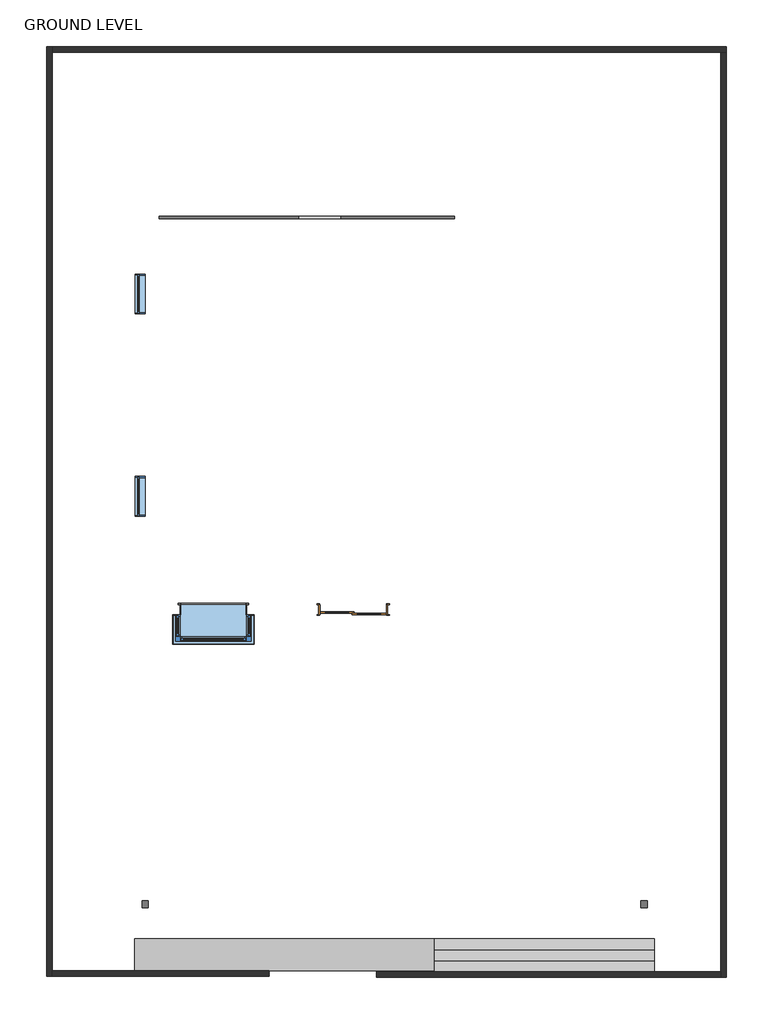
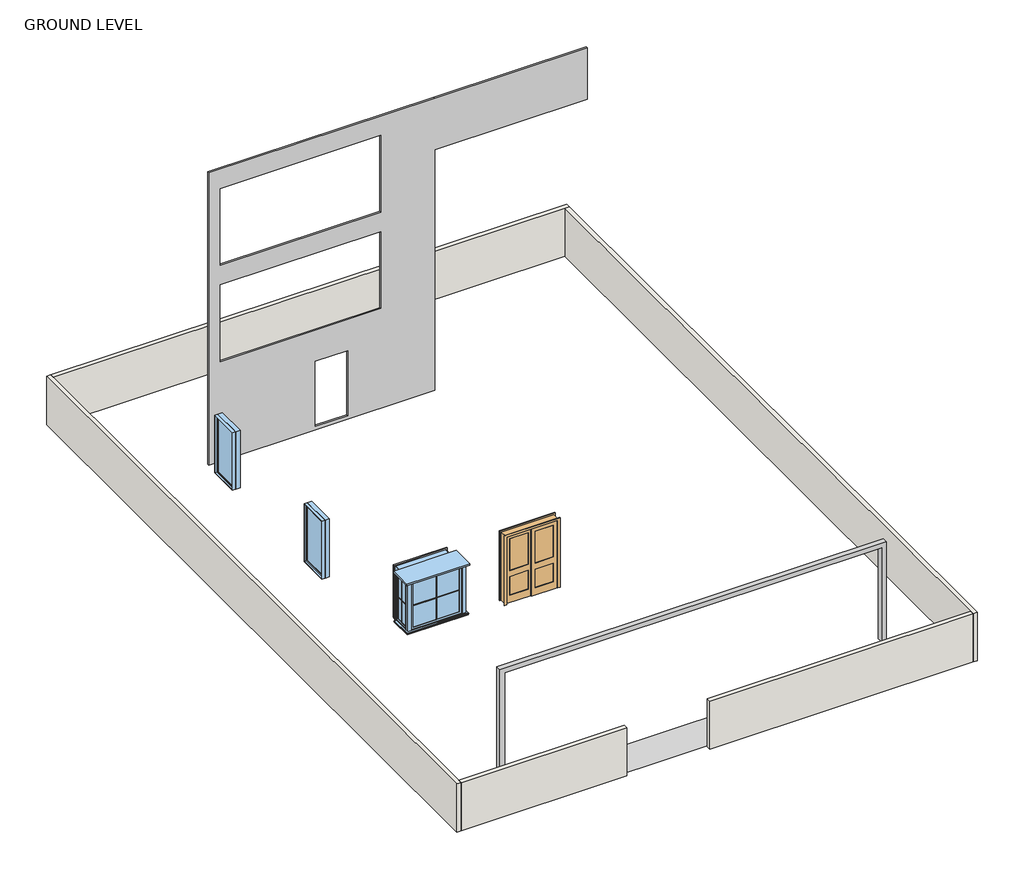
# One storey: 8 proxies, 5 walls, 3 windows, 1 door.
"""IFC4 building model written with IfcOpenShell, lengths in millimetres."""

from ifc_helpers import new_model, si_unit, origin, origin_with_axes, place, context, project, spatial, polyline, outline, extrude, faceted_brep, transform, mapped, element, save
from components import generic_models_11_generic_models_11_747a53b2, generic_models_19_generic_models_19_d8e6bd8f, generic_models_30_generic_models_30_d6d6d2d1, generic_models_31_generic_models_31_aad501af, muntin_pattern_2x2_muntin_pattern_2x2_eeef18e2, muntin_pattern_2x2_muntin_pattern_2x2_218eda85, trim_window_interior_flat_picture_frame_524b5c54, door_2b3f2951, window_2e8ca8a3, window_dda79932

model = new_model("IFC4")

# Units and contexts
model_context = context("Model", 3, world=origin())
ifc_project = project(units=[si_unit("LENGTHUNIT", "METRE", prefix="MILLI")], contexts=[model_context])

# Site, building, storey
site = spatial("IfcSite", under=ifc_project)
building = spatial("IfcBuilding", under=site)
storey = spatial("IfcBuildingStorey", under=building, Name="GROUND LEVEL", Elevation=0.0)

# Proxies
placement = place(None, origin())
generic_models_11_generic_models_11_shape = generic_models_11_generic_models_11_747a53b2(model_context)
element("IfcBuildingElementProxy", 1, Name="Generic Models 11 : Generic Models 11", ObjectType="Generic Models 11 : Generic Models 11", at=placement, inside=storey, context=model_context, shape_type="MappedRepresentation", body=[
    mapped(generic_models_11_generic_models_11_shape, transform((0.0, 0.0, 0.0), x_axis=(1.0, 0.0, 0.0), y_axis=(0.0, 1.0, 0.0), z_axis=(0.0, 0.0, 1.0))),
])
generic_models_19_generic_models_19_shape = generic_models_19_generic_models_19_d8e6bd8f(model_context)
element("IfcBuildingElementProxy", 2, Name="Generic Models 19 : Generic Models 19", ObjectType="Generic Models 19 : Generic Models 19", at=placement, inside=storey, context=model_context, shape_type="MappedRepresentation", body=[
    mapped(generic_models_19_generic_models_19_shape, transform((0.0, 0.0, 0.0), x_axis=(1.0, 0.0, 0.0), y_axis=(0.0, 1.0, 0.0), z_axis=(0.0, 0.0, 1.0))),
])
generic_models_30_generic_models_30_shape = generic_models_30_generic_models_30_d6d6d2d1(model_context)
element("IfcBuildingElementProxy", 3, Name="Generic Models 30 : Generic Models 30", ObjectType="Generic Models 30 : Generic Models 30", at=placement, inside=storey, context=model_context, shape_type="MappedRepresentation", body=[
    mapped(generic_models_30_generic_models_30_shape, transform((0.0, 0.0, 0.0), x_axis=(1.0, 0.0, 0.0), y_axis=(0.0, 1.0, 0.0), z_axis=(0.0, 0.0, 1.0))),
])
generic_models_31_generic_models_31_shape = generic_models_31_generic_models_31_aad501af(model_context)
element("IfcBuildingElementProxy", 4, Name="Generic Models 31 : Generic Models 31", ObjectType="Generic Models 31 : Generic Models 31", at=placement, inside=storey, context=model_context, shape_type="MappedRepresentation", body=[
    mapped(generic_models_31_generic_models_31_shape, transform((0.0, 0.0, 0.0), x_axis=(1.0, 0.0, 0.0), y_axis=(0.0, 1.0, 0.0), z_axis=(0.0, 0.0, 1.0))),
])
muntin_pattern_2x2_muntin_pattern_2x2_shape = muntin_pattern_2x2_muntin_pattern_2x2_eeef18e2(model_context)
element("IfcBuildingElementProxy", 5, Name="Muntin Pattern_2x2 : Muntin Pattern_2x2", ObjectType="Muntin Pattern_2x2 : Muntin Pattern_2x2", at=placement, inside=storey, context=model_context, shape_type="MappedRepresentation", body=[
    mapped(muntin_pattern_2x2_muntin_pattern_2x2_shape, transform((-8201.8781265, -1299.9392532, 730.25), x_axis=(-1.0, 0.0, 0.0), y_axis=(0.0, -1.0, 0.0), z_axis=(0.0, 0.0, 1.0))),
])
muntin_pattern_2x2_muntin_pattern_2x2_2_shape = muntin_pattern_2x2_muntin_pattern_2x2_218eda85(model_context)
element("IfcBuildingElementProxy", 6, Name="Muntin Pattern_2x2 : Muntin Pattern_2x2", ObjectType="Muntin Pattern_2x2 : Muntin Pattern_2x2", at=placement, inside=storey, context=model_context, shape_type="MappedRepresentation", body=[
    mapped(muntin_pattern_2x2_muntin_pattern_2x2_2_shape, transform((-7379.5531265, -985.6142532, 730.25), x_axis=(0.0, 1.0, 0.0), y_axis=(-1.0, 0.0, 0.0), z_axis=(0.0, 0.0, 1.0))),
])
element("IfcBuildingElementProxy", 7, Name="Muntin Pattern_2x2 : Muntin Pattern_2x2", ObjectType="Muntin Pattern_2x2 : Muntin Pattern_2x2", at=placement, inside=storey, context=model_context, shape_type="MappedRepresentation", body=[
    mapped(muntin_pattern_2x2_muntin_pattern_2x2_2_shape, transform((-9024.2031265, -985.6142532, 730.25), x_axis=(0.0, -1.0, 0.0), y_axis=(1.0, 0.0, 0.0), z_axis=(0.0, 0.0, 1.0))),
])
trim_window_interior_flat_picture_frame_shape = trim_window_interior_flat_picture_frame_524b5c54(model_context)
element("IfcBuildingElementProxy", 8, Name="Trim-Window-Interior-Flat : Picture Frame", ObjectType="Trim-Window-Interior-Flat : Picture Frame", at=placement, inside=storey, context=model_context, shape_type="MappedRepresentation", body=[
    mapped(trim_window_interior_flat_picture_frame_shape, transform((-8201.8781265, -503.0142532, 2184.4), x_axis=(-1.0, 0.0, 0.0), y_axis=(0.0, 0.0, 1.0), z_axis=(0.0, 1.0, 0.0))),
])

# Door
door_shape = door_2b3f2951(model_context)
element("IfcDoor", 9, ObjectType="Door-Interior-Double-Sliding-2_Panel-Wood : 60\" x 84\"", at=placement, inside=storey, context=model_context, shape_type="MappedRepresentation", body=[
    mapped(door_shape, transform((-5001.4781265, -620.4892532, 0.0), x_axis=(-1.0, 0.0, 0.0), y_axis=(0.0, -1.0, 0.0), z_axis=(0.0, 0.0, 1.0))),
])

# Walls
element("IfcWall", 10, ObjectType="parapet wall 5\"", at=placement, inside=storey, context=model_context, shape_type="Brep", body=[
    faceted_brep([(-11897.5781265, -9005.1279205, 0.0), (-11897.5781265, -8878.1279205, 0.0), (-11897.5781265, 12146.1857468, 0.0), (-11897.5781265, 12273.1857468, 0.0), (-11897.5781265, 12273.1857468, 1524.0), (-11897.5781265, 12146.1857468, 1524.0), (-11897.5781265, -8878.1279205, 1524.0), (-11897.5781265, -9005.1279205, 1524.0), (-12024.5781265, -9005.1279205, 0.0), (-12024.5781265, -9005.1279205, 1524.0), (-12024.5781265, 12273.1857468, 1524.0), (-12024.5781265, 12273.1857468, 0.0)], [[[0, 1, 2, 3, 4, 5, 6, 7]], [[8, 9, 10, 11]], [[3, 2, 1, 0, 8, 11]], [[7, 6, 5, 4, 10, 9]], [[4, 3, 11, 10]], [[0, 7, 9, 8]]]),
])
element("IfcWall", 11, ObjectType="parapet wall 5\"", at=placement, inside=storey, context=model_context, shape_type="Brep", body=[
    faceted_brep([(-11897.5781265, 12146.1857468, 0.0), (3418.6218735, 12146.1857468, 0.0), (3545.6218735, 12146.1857468, 0.0), (3545.6218735, 12146.1857468, 1524.0), (3418.6218735, 12146.1857468, 1524.0), (-11897.5781265, 12146.1857468, 1524.0), (-11897.5781265, 12273.1857468, 0.0), (-11897.5781265, 12273.1857468, 1524.0), (3545.6218735, 12273.1857468, 1524.0), (3545.6218735, 12273.1857468, 0.0)], [[[0, 1, 2, 3, 4, 5]], [[6, 7, 8, 9]], [[2, 1, 0, 6, 9]], [[5, 4, 3, 8, 7]], [[0, 5, 7, 6]], [[3, 2, 9, 8]]]),
])
element("IfcWall", 12, ObjectType="parapet wall 5\"", at=placement, inside=storey, context=model_context, shape_type="Brep", body=[
    faceted_brep([(3418.6218735, 12146.1857468, 0.0), (3418.6218735, -8909.9432518, 0.0), (3418.6218735, -9036.9432518, 0.0), (3418.6218735, -9036.9432518, 1524.0), (3418.6218735, -8909.9432518, 1524.0), (3418.6218735, 12146.1857468, 1524.0), (3545.6218735, 12146.1857468, 0.0), (3545.6218735, 12146.1857468, 1524.0), (3545.6218735, -9036.9432518, 1524.0), (3545.6218735, -9036.9432518, 0.0)], [[[0, 1, 2, 3, 4, 5]], [[6, 7, 8, 9]], [[2, 1, 0, 6, 9]], [[5, 4, 3, 8, 7]], [[0, 5, 7, 6]], [[3, 2, 9, 8]]]),
])
element("IfcWall", 13, ObjectType="parapet wall 5\"", at=placement, inside=storey, context=model_context, shape_type="SweptSolid", body=[
    extrude(outline(polyline([(-4468.0781265, -8909.9432518), (3418.6218735, -8909.9432518), (3418.6218735, -9036.9432518), (-4468.0781265, -9036.9432518), (-4468.0781265, -8909.9432518)])), origin_with_axes(), (0.0, 0.0, 1.0), 1524.0),
])
element("IfcWall", 14, ObjectType="parapet wall 5\"", at=placement, inside=storey, context=model_context, shape_type="SweptSolid", body=[
    extrude(outline(polyline([(-11897.5781265, -8878.1279205), (-6931.8781265, -8878.1279205), (-6931.8781265, -9005.1279205), (-11897.5781265, -9005.1279205), (-11897.5781265, -8878.1279205)])), origin_with_axes(), (0.0, 0.0, 1.0), 1524.0),
])

# Windows
window_shape = window_2e8ca8a3(model_context)
element("IfcWindow", 15, ObjectType="Fixed : window 3' x 6\"", at=placement, inside=storey, context=model_context, shape_type="MappedRepresentation", body=[
    mapped(window_shape, transform((-9878.2781265, 6647.0857468, 0.0), x_axis=(0.0, 1.0, 0.0), y_axis=(-1.0, 0.0, 0.0), z_axis=(0.0, 0.0, 1.0))),
])
element("IfcWindow", 16, ObjectType="Fixed : window 3' x 6\"", at=placement, inside=storey, context=model_context, shape_type="MappedRepresentation", body=[
    mapped(window_shape, transform((-9878.2781265, 2011.5857468, 0.0), x_axis=(0.0, 1.0, 0.0), y_axis=(-1.0, 0.0, 0.0), z_axis=(0.0, 0.0, 1.0))),
])
window_2_shape = window_dda79932(model_context)
element("IfcWindow", 17, ObjectType="Window-Bay-Casement-Box-90_Degree_Angle-Center_Fixed : 60\" x 60\" x 24\"", at=placement, inside=storey, context=model_context, shape_type="MappedRepresentation", body=[
    mapped(window_2_shape, transform((-8201.8781265, -617.3142532, 0.0), x_axis=(-1.0, 0.0, 0.0), y_axis=(0.0, -1.0, 0.0), z_axis=(0.0, 0.0, 1.0))),
])

save(model, "model.ifc")

# Revit data of these elements
# Type "Muntin Pattern_2x2 : Muntin Pattern_2x2"
#   Width [instance default] = 4' - 0"
#   Thickness = 0' - 0 1/2"
#   Height [instance default] = 4' - 0"
#   Distance = 0' - 0 3/4"
#   Interior Material [instance default] = none
#   Exterior Material [instance default] = none
#   Default Elevation = 0
# Type "Trim-Window-Interior-Flat : Picture Frame"
#   Trim Thickness_Picture Frame = 0' - 1 1/4"
#   Trim Width = 0' - 2 1/4"
#   Trim Thickness_with Sill = 0' - 0 3/4"
#   Sill Thickness = 0' - 1 1/4"
#   Opening Width [instance default] = 2' - 0"
#   Opening Height [instance default] = 3' - 0"
#   Default Elevation = 4' - 0"
#   Sill = no
#   Picture Frame = yes
#   Trim Material [instance default] = none
# Type "Door-Interior-Double-Sliding-2_Panel-Wood : 60\" x 84\""
#   Type Mark = "10"
#   Assembly Code = "C1020300"
#   Analytic Construction = "Wooden"
#   Top Rail = 0' - 4 11/16"
#   Thickness = 0' - 1 3/8"
#   Thermal Resistance (R) = 2.5876 (h·ft²·°F)/BTU
#   Stiles = 0' - 4 3/4"
#   Rough Width = 5' - 2"
#   Rough Height = 7' - 1"
#   Lock Rail = 0' - 7 1/2"
#   Height = 7' - 0"
#   Width = 5' - 0"
#   Heat Transfer Coefficient (U) = 0.3865 BTU/(h·ft²·°F)
#   Bottom Rail = 0' - 9 1/8"
#   Trim Material = Cherry
#   Panel Material = Cherry
#   Frame Material = Cherry
#   Visual Light Transmittance = 0
#   Solar Heat Gain Coefficient = 0
#   Wall Closure = (empty or 0)
#   Function = (empty or 0)
# Type "parapet wall 5\""
#   Assembly Code = "B2010"
# Type "Fixed : window 3' x 6\""
#   Type Mark = "26"
#   Construction Type Id = "GSP4R"
#   Assembly Code = "B2020100"
#   Analytic Construction = "1/8 in Pilkington single glazing"
#   Visual Light Transmittance = 0.9
#   Solar Heat Gain Coefficient = 0.78
#   Heat Transfer Coefficient (U) = 0.6496 BTU/(h·ft²·°F)
#   Height = 6' - 0"
#   Default Sill Height = 3' - 0"
#   Width = 3' - 0"
#   Window Inset = 0' - 2"
#   Define Thermal Properties by = 1
#   Glass Pane Material = Glass
#   Sash Material = Sash
#   Wall Closure = (empty or 0)
# Type "Window-Bay-Casement-Box-90_Degree_Angle-Center_Fixed : 60\" x 60\" x 24\""
#   Type Mark = "29"
#   Fire Rating = "0.5h"
#   Assembly Code = "B2020100"
#   Analytic Construction = "1/8 in Pilkington single glazing"
#   Width = 5' - 0"
#   Wall Thickness [instance default] = 0' - 6"
#   Visual Light Transmittance = 0.9
#   Trim Width = 5' - 8"
#   Trim Height = 5' - 0"
#   Thermal Resistance (R) = 1.5394 (h·ft²·°F)/BTU
#   Solar Heat Gain Coefficient = 0.86
#   Rough Width = 5' - 0 1/2"
#   Rough Height = 5' - 0 1/2"
#   Height 1 = 5' - 2"
#   Height = 5' - 0"
#   Heat Transfer Coefficient (U) = 0.6496 BTU/(h·ft²·°F)
#   Depth = 2' - 0"
#   Default Sill Height = 2' - 0"
#   Side Muntin Visibility = yes
#   Center Muntin Visibility = yes
#   Interior Trim Visibility [instance default] = yes
#   Exterior Trim Visibility [instance default] = yes
#   Side Muntin Pattern = Muntin Pattern_2x2 : Muntin Pattern_2x2
#   Center Muntin Pattern = Muntin Pattern_2x2 : Muntin Pattern_2x2
#   Interior Trim Material = Wood - Stained
#   Exterior Trim Material = Clad - White
#   Exterior Trim = element 424880
#   Interior Trim = Trim-Window-Interior-Flat : Picture Frame
#   Interior Frame Material = Wood - Stained
#   Glass Panel Material = Glass
#   Exterior Frame Material = Clad - White
#   Wall Closure = (empty or 0)
# Element 1 (IfcBuildingElementProxy, "Generic Models 11 : Generic Models 11")
#   Phase Created = New Construction
# Element 2 (IfcBuildingElementProxy, "Generic Models 19 : Generic Models 19")
#   Phase Created = New Construction
# Element 3 (IfcBuildingElementProxy, "Generic Models 30 : Generic Models 30")
#   Phase Created = New Construction
# Element 4 (IfcBuildingElementProxy, "Generic Models 31 : Generic Models 31")
#   Phase Created = New Construction
# Element 5 (IfcBuildingElementProxy, "Muntin Pattern_2x2 : Muntin Pattern_2x2")
#   Width = 4' - 6 1/2"
#   Height = 4' - 6 1/2"
#   Interior Material = Wood - Stained
#   Exterior Material = Clad - White
#   Phase Created = New Construction
#   Materials on its faces: "Clad - White", "Wood - Stained"
# Elements 6, 7 (IfcBuildingElementProxy, "Muntin Pattern_2x2 : Muntin Pattern_2x2")
#   Width = 1' - 2 1/2"
#   Height = 4' - 6 1/2"
#   Interior Material = Wood - Stained
#   Exterior Material = Clad - White
#   Phase Created = New Construction
#   Materials on its faces: "Clad - White", "Wood - Stained"
# Element 8 (IfcBuildingElementProxy, "Trim-Window-Interior-Flat : Picture Frame")
#   Opening Width = 5' - 0"
#   Opening Height = 5' - 2"
#   Trim Material = Wood - Stained
#   Phase Created = New Construction
#   Materials on its faces: "Wood - Stained"
# Element 9 (IfcDoor, "Door-Interior-Double-Sliding-2_Panel-Wood : 60\" x 84\"")
#   Phase Created = New Construction
#   Materials on its faces: "Cherry"
# Elements 10, 11, 12, 13, 14 (IfcWall, "parapet wall 5\"")
#   Top Offset = 0' - 0"
#   Base Offset = 0' - 0"
#   Unconnected Height = 5' - 0"
#   wall height = 5' - 0"
#   Phase Created = New Construction
#   Base Constraint = GROUND LEVEL
# Element 15 (IfcWindow, "Fixed : window 3' x 6\"")
#   Mark = "13"
#   Phase Created = New Construction
#   Materials on its faces: "Sash", "Glass"
# Element 16 (IfcWindow, "Fixed : window 3' x 6\"")
#   Mark = "14"
#   Phase Created = New Construction
#   Materials on its faces: "Sash", "Glass"
# Element 17 (IfcWindow, "Window-Bay-Casement-Box-90_Degree_Angle-Center_Fixed : 60\" x 60\" x 24\"")
#   Mark = "30"
#   Interior Trim Visibility = yes
#   Exterior Trim Visibility = yes
#   Phase Created = New Construction
#   Materials on its faces: "Clad - White", "Wood - Stained", "Glass"
# Materials
#   "Cherry": class "Wood", colour RGB 226 177 128, transparency 0, Description = "Prunus Serotina", Cost = 0
#   "Glass": class "Glass", colour RGB 0 128 192, transparency 0.75, Description = "Soda Lime Glass", Cost = 0
#   "Sash": class "Wood", colour RGB 224 178 126, transparency 0, Cost = 0
#   "Wood - Stained": class "Wood", colour RGB 224 178 126, transparency 0, Cost = 0
#   "Clad - White": class "Wood", colour RGB 242 242 238, transparency 0, Cost = 0
# Room, not placed, phase "New Construction", upper offset 0' - 0", lower offset 0' - 0"
#   Number = "1"
#   Name = "Room"
